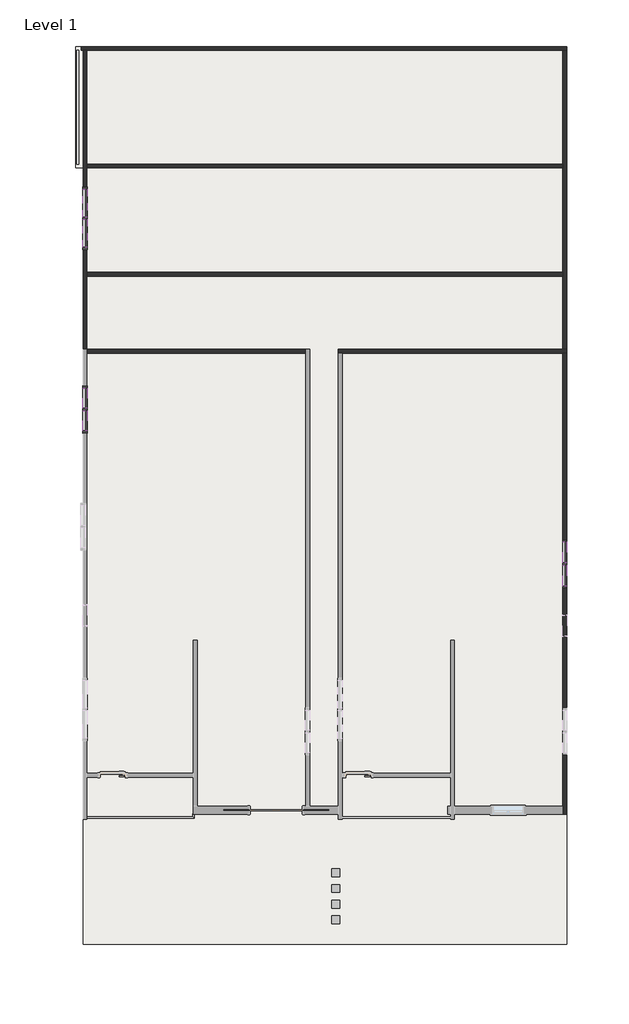
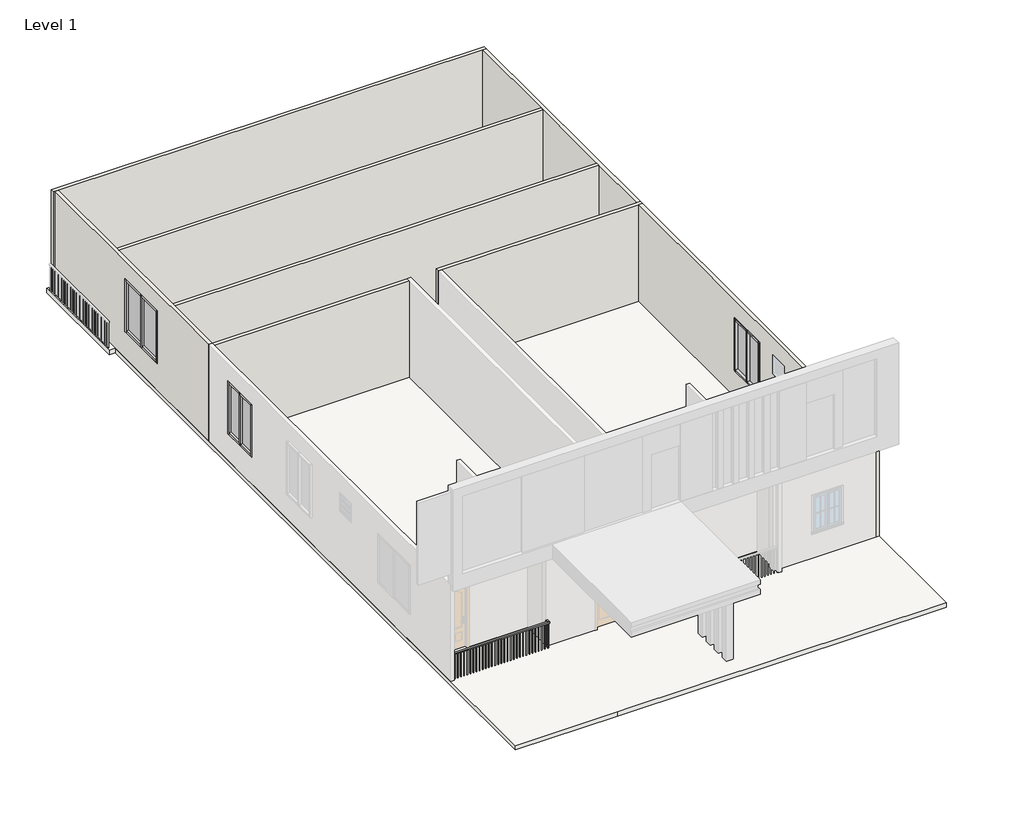
# One storey, part 2 of 3: 21 members, 8 walls, 6 plates, 1 railing, 1 slab.
"""IFC4 building model written with IfcOpenShell, lengths in millimetres."""

from ifc_helpers import new_model, si_unit, frame, origin, origin_with_axes, place, context, project, spatial, polyline, outline, extrude, faceted_brep, transform, mapped, element, save
from components import member_3f0e0172, member_96ae0c19, member_d60e8053, member_2fae0574, member_3e1d4a65, system_panel_glazed_c4393626, system_panel_glazed_d2c73f4b, system_panel_glazed_30879ba3

model = new_model("IFC4")

# Units and contexts
model_context = context("Model", 3, world=origin())
ifc_project = project(units=[si_unit("LENGTHUNIT", "METRE", prefix="MILLI")], contexts=[model_context])

# Site, building, storey
site = spatial("IfcSite", under=ifc_project)
building = spatial("IfcBuilding", under=site)
storey = spatial("IfcBuildingStorey", under=building, Name="Level 1", Elevation=0.0)

# Members
placement = place(None, origin())
member_shape = member_3f0e0172(model_context)
element("IfcMember", 1, ObjectType="Rectangular Mullion : 2.5\" x 5\" rectangular", at=placement, inside=storey, context=model_context, shape_type="MappedRepresentation", body=[
    mapped(member_shape, transform((5848.1708786, -3933.7021821, 2743.2), x_axis=(0.0, 0.0, 1.0), y_axis=(-1.0, 0.0, 0.0), z_axis=(0.0, -1.0, 0.0))),
])
element("IfcMember", 2, ObjectType="Rectangular Mullion : 2.5\" x 5\" rectangular", at=placement, inside=storey, context=model_context, shape_type="MappedRepresentation", body=[
    mapped(member_shape, transform((5848.1708786, -3254.2521821, 2743.2), x_axis=(0.0, 0.0, 1.0), y_axis=(-1.0, 0.0, 0.0), z_axis=(0.0, -1.0, 0.0))),
])
element("IfcMember", 3, ObjectType="Rectangular Mullion : 2.5\" x 5\" rectangular", at=placement, inside=storey, context=model_context, shape_type="MappedRepresentation", body=[
    mapped(member_shape, transform((5848.1708786, -2638.3021821, 914.4), x_axis=(0.0, 0.0, -1.0), y_axis=(-1.0, 0.0, 0.0), z_axis=(0.0, 1.0, 0.0))),
])
element("IfcMember", 4, ObjectType="Rectangular Mullion : 2.5\" x 5\" rectangular", at=placement, inside=storey, context=model_context, shape_type="MappedRepresentation", body=[
    mapped(member_shape, transform((5848.1708786, -3317.7521821, 914.4), x_axis=(0.0, 0.0, -1.0), y_axis=(-1.0, 0.0, 0.0), z_axis=(0.0, 1.0, 0.0))),
])
member_2_shape = member_96ae0c19(model_context)
element("IfcMember", 5, ObjectType="Rectangular Mullion : 2.5\" x 5\" rectangular", at=placement, inside=storey, context=model_context, shape_type="MappedRepresentation", body=[
    mapped(member_2_shape, transform((-8153.157583, 600.1666267, 2743.2), x_axis=(0.0, 0.0, 1.0), y_axis=(-1.0, 0.0, 0.0), z_axis=(0.0, -1.0, 0.0))),
])
element("IfcMember", 6, ObjectType="Rectangular Mullion : 2.5\" x 5\" rectangular", at=placement, inside=storey, context=model_context, shape_type="MappedRepresentation", body=[
    mapped(member_2_shape, transform((-8153.157583, 1254.9937905, 2743.2), x_axis=(0.0, 0.0, 1.0), y_axis=(-1.0, 0.0, 0.0), z_axis=(0.0, -1.0, 0.0))),
])
element("IfcMember", 7, ObjectType="Rectangular Mullion : 2.5\" x 5\" rectangular", at=placement, inside=storey, context=model_context, shape_type="MappedRepresentation", body=[
    mapped(member_2_shape, transform((-8153.157583, 1846.3209543, 914.4), x_axis=(0.0, 0.0, -1.0), y_axis=(-1.0, 0.0, 0.0), z_axis=(0.0, 1.0, 0.0))),
])
element("IfcMember", 8, ObjectType="Rectangular Mullion : 2.5\" x 5\" rectangular", at=placement, inside=storey, context=model_context, shape_type="MappedRepresentation", body=[
    mapped(member_2_shape, transform((-8153.157583, 1191.4937905, 914.4), x_axis=(0.0, 0.0, -1.0), y_axis=(-1.0, 0.0, 0.0), z_axis=(0.0, 1.0, 0.0))),
])
member_3_shape = member_d60e8053(model_context)
element("IfcMember", 9, ObjectType="Rectangular Mullion : 2.5\" x 5\" rectangular", at=placement, inside=storey, context=model_context, shape_type="MappedRepresentation", body=[
    mapped(member_3_shape, transform((5848.1708786, -3286.0021821, 914.4), x_axis=(0.0, -1.0, 0.0), y_axis=(-1.0, 0.0, 0.0), z_axis=(0.0, 0.0, -1.0))),
])
element("IfcMember", 10, ObjectType="Rectangular Mullion : 2.5\" x 5\" rectangular", at=placement, inside=storey, context=model_context, shape_type="MappedRepresentation", body=[
    mapped(member_3_shape, transform((-8153.157583, 1223.2437905, 914.4), x_axis=(0.0, -1.0, 0.0), y_axis=(-1.0, 0.0, 0.0), z_axis=(0.0, 0.0, -1.0))),
])
element("IfcMember", 11, ObjectType="Rectangular Mullion : 2.5\" x 5\" rectangular", at=placement, inside=storey, context=model_context, shape_type="MappedRepresentation", body=[
    mapped(member_3_shape, transform((-8153.157583, 6807.1511393, 914.4), x_axis=(0.0, -1.0, 0.0), y_axis=(-1.0, 0.0, 0.0), z_axis=(0.0, 0.0, -1.0))),
])
member_4_shape = member_2fae0574(model_context)
element("IfcMember", 12, ObjectType="Rectangular Mullion : 2.5\" x 5\" rectangular", at=placement, inside=storey, context=model_context, shape_type="MappedRepresentation", body=[
    mapped(member_4_shape, transform((5848.1708786, -2574.8021821, 2743.2), x_axis=(0.0, 1.0, 0.0), y_axis=(-1.0, 0.0, 0.0), z_axis=(0.0, 0.0, 1.0))),
])
element("IfcMember", 13, ObjectType="Rectangular Mullion : 2.5\" x 5\" rectangular", at=placement, inside=storey, context=model_context, shape_type="MappedRepresentation", body=[
    mapped(member_4_shape, transform((-8153.157583, 1909.8209543, 2743.2), x_axis=(0.0, 1.0, 0.0), y_axis=(-1.0, 0.0, 0.0), z_axis=(0.0, 0.0, 1.0))),
])
element("IfcMember", 14, ObjectType="Rectangular Mullion : 2.5\" x 5\" rectangular", at=placement, inside=storey, context=model_context, shape_type="MappedRepresentation", body=[
    mapped(member_4_shape, transform((-8153.157583, 7721.9533991, 2743.2), x_axis=(0.0, 1.0, 0.0), y_axis=(-1.0, 0.0, 0.0), z_axis=(0.0, 0.0, 1.0))),
])
element("IfcMember", 15, ObjectType="Rectangular Mullion : 2.5\" x 5\" rectangular", at=placement, inside=storey, context=model_context, shape_type="MappedRepresentation", body=[
    mapped(member_4_shape, transform((5848.1708786, -3997.2021821, 914.4), x_axis=(0.0, -1.0, 0.0), y_axis=(-1.0, 0.0, 0.0), z_axis=(0.0, 0.0, -1.0))),
])
element("IfcMember", 16, ObjectType="Rectangular Mullion : 2.5\" x 5\" rectangular", at=placement, inside=storey, context=model_context, shape_type="MappedRepresentation", body=[
    mapped(member_4_shape, transform((-8153.157583, 536.6666267, 914.4), x_axis=(0.0, -1.0, 0.0), y_axis=(-1.0, 0.0, 0.0), z_axis=(0.0, 0.0, -1.0))),
])
element("IfcMember", 17, ObjectType="Rectangular Mullion : 2.5\" x 5\" rectangular", at=placement, inside=storey, context=model_context, shape_type="MappedRepresentation", body=[
    mapped(member_4_shape, transform((-8153.157583, 5892.3488795, 914.4), x_axis=(0.0, -1.0, 0.0), y_axis=(-1.0, 0.0, 0.0), z_axis=(0.0, 0.0, -1.0))),
])
member_5_shape = member_3e1d4a65(model_context)
element("IfcMember", 18, ObjectType="Rectangular Mullion : 2.5\" x 5\" rectangular", at=placement, inside=storey, context=model_context, shape_type="MappedRepresentation", body=[
    mapped(member_5_shape, transform((-8153.157583, 5955.8488795, 2743.2), x_axis=(0.0, 0.0, 1.0), y_axis=(-1.0, 0.0, 0.0), z_axis=(0.0, -1.0, 0.0))),
])
element("IfcMember", 19, ObjectType="Rectangular Mullion : 2.5\" x 5\" rectangular", at=placement, inside=storey, context=model_context, shape_type="MappedRepresentation", body=[
    mapped(member_5_shape, transform((-8153.157583, 6838.9011393, 2743.2), x_axis=(0.0, 0.0, 1.0), y_axis=(-1.0, 0.0, 0.0), z_axis=(0.0, -1.0, 0.0))),
])
element("IfcMember", 20, ObjectType="Rectangular Mullion : 2.5\" x 5\" rectangular", at=placement, inside=storey, context=model_context, shape_type="MappedRepresentation", body=[
    mapped(member_5_shape, transform((-8153.157583, 7658.4533991, 914.4), x_axis=(0.0, 0.0, -1.0), y_axis=(-1.0, 0.0, 0.0), z_axis=(0.0, 1.0, 0.0))),
])
element("IfcMember", 21, ObjectType="Rectangular Mullion : 2.5\" x 5\" rectangular", at=placement, inside=storey, context=model_context, shape_type="MappedRepresentation", body=[
    mapped(member_5_shape, transform((-8153.157583, 6775.4011393, 914.4), x_axis=(0.0, 0.0, -1.0), y_axis=(-1.0, 0.0, 0.0), z_axis=(0.0, 1.0, 0.0))),
])

# Plates
system_panel_glazed_shape = system_panel_glazed_c4393626(model_context)
element("IfcPlate", 22, ObjectType="System Panel : Glazed", at=placement, inside=storey, context=model_context, shape_type="MappedRepresentation", body=[
    mapped(system_panel_glazed_shape, transform((-8153.157583, 1550.6573724, 977.9), x_axis=(0.0, -1.0, 0.0), y_axis=(1.0, 0.0, 0.0), z_axis=(0.0, 0.0, 1.0))),
])
element("IfcPlate", 23, ObjectType="System Panel : Glazed", at=placement, inside=storey, context=model_context, shape_type="MappedRepresentation", body=[
    mapped(system_panel_glazed_shape, transform((-8153.157583, 895.8302086, 977.9), x_axis=(0.0, -1.0, 0.0), y_axis=(1.0, 0.0, 0.0), z_axis=(0.0, 0.0, 1.0))),
])
system_panel_glazed_2_shape = system_panel_glazed_d2c73f4b(model_context)
element("IfcPlate", 24, ObjectType="System Panel : Glazed", at=placement, inside=storey, context=model_context, shape_type="MappedRepresentation", body=[
    mapped(system_panel_glazed_2_shape, transform((5848.1708786, -2946.2771821, 977.9), x_axis=(0.0, -1.0, 0.0), y_axis=(1.0, 0.0, 0.0), z_axis=(0.0, 0.0, 1.0))),
])
element("IfcPlate", 25, ObjectType="System Panel : Glazed", at=placement, inside=storey, context=model_context, shape_type="MappedRepresentation", body=[
    mapped(system_panel_glazed_2_shape, transform((5848.1708786, -3625.7271821, 977.9), x_axis=(0.0, -1.0, 0.0), y_axis=(1.0, 0.0, 0.0), z_axis=(0.0, 0.0, 1.0))),
])
system_panel_glazed_3_shape = system_panel_glazed_30879ba3(model_context)
element("IfcPlate", 26, ObjectType="System Panel : Glazed", at=placement, inside=storey, context=model_context, shape_type="MappedRepresentation", body=[
    mapped(system_panel_glazed_3_shape, transform((-8153.157583, 7248.6772692, 977.9), x_axis=(0.0, -1.0, 0.0), y_axis=(1.0, 0.0, 0.0), z_axis=(0.0, 0.0, 1.0))),
])
element("IfcPlate", 27, ObjectType="System Panel : Glazed", at=placement, inside=storey, context=model_context, shape_type="MappedRepresentation", body=[
    mapped(system_panel_glazed_3_shape, transform((-8153.157583, 6365.6250094, 977.9), x_axis=(0.0, -1.0, 0.0), y_axis=(1.0, 0.0, 0.0), z_axis=(0.0, 0.0, 1.0))),
])

# Railing
element("IfcRailing", 28, ObjectType="Handrail - Rectangular", at=placement, inside=storey, context=model_context, shape_type="SolidModel", body=[
    faceted_brep([(-8153.157583, -10659.0005933, 914.4), (-8153.157583, -10659.0005933, 863.6), (-8153.157583, -10709.8005933, 863.6), (-8153.157583, -10709.8005933, 914.4), (-5014.0237038, -10659.0005933, 914.4), (-5014.0237038, -10659.0005933, 863.6), (-4963.2237038, -10709.8005933, 863.6), (-4963.2237038, -10709.8005933, 914.4), (-5014.0237038, -10582.0742041, 914.4), (-4963.2237038, -10582.0742041, 914.4), (-4963.2237038, -10582.0742041, 863.6), (-5014.0237038, -10582.0742041, 863.6)], [[[0, 1, 2, 3]], [[1, 0, 4, 5]], [[2, 1, 5, 6]], [[3, 2, 6, 7]], [[0, 3, 7, 4]], [[8, 9, 10, 11]], [[5, 4, 8, 11]], [[6, 5, 11, 10]], [[7, 6, 10, 9]], [[4, 7, 9, 8]]]),
    extrude(outline(polyline([(-4979.0987038, -10592.3255933), (-4998.1487038, -10592.3255933), (-4998.1487038, -10573.2755933), (-4979.0987038, -10573.2755933), (-4979.0987038, -10592.3255933)])), origin_with_axes(), (0.0, 0.0, 1.0), 863.6),
    extrude(outline(polyline([(-5013.082583, -10693.9255933), (-5013.082583, -10674.8755933), (-4994.032583, -10674.8755933), (-4994.032583, -10693.9255933), (-5013.082583, -10693.9255933)])), origin_with_axes(), (0.0, 0.0, 1.0), 863.6),
    extrude(outline(polyline([(-5114.682583, -10693.9255933), (-5114.682583, -10674.8755933), (-5095.632583, -10674.8755933), (-5095.632583, -10693.9255933), (-5114.682583, -10693.9255933)])), origin_with_axes(), (0.0, 0.0, 1.0), 863.6),
    extrude(outline(polyline([(-5216.282583, -10693.9255933), (-5216.282583, -10674.8755933), (-5197.232583, -10674.8755933), (-5197.232583, -10693.9255933), (-5216.282583, -10693.9255933)])), origin_with_axes(), (0.0, 0.0, 1.0), 863.6),
    extrude(outline(polyline([(-5317.882583, -10693.9255933), (-5317.882583, -10674.8755933), (-5298.832583, -10674.8755933), (-5298.832583, -10693.9255933), (-5317.882583, -10693.9255933)])), origin_with_axes(), (0.0, 0.0, 1.0), 863.6),
    extrude(outline(polyline([(-5419.482583, -10693.9255933), (-5419.482583, -10674.8755933), (-5400.432583, -10674.8755933), (-5400.432583, -10693.9255933), (-5419.482583, -10693.9255933)])), origin_with_axes(), (0.0, 0.0, 1.0), 863.6),
    extrude(outline(polyline([(-5521.082583, -10693.9255933), (-5521.082583, -10674.8755933), (-5502.032583, -10674.8755933), (-5502.032583, -10693.9255933), (-5521.082583, -10693.9255933)])), origin_with_axes(), (0.0, 0.0, 1.0), 863.6),
    extrude(outline(polyline([(-5622.682583, -10693.9255933), (-5622.682583, -10674.8755933), (-5603.632583, -10674.8755933), (-5603.632583, -10693.9255933), (-5622.682583, -10693.9255933)])), origin_with_axes(), (0.0, 0.0, 1.0), 863.6),
    extrude(outline(polyline([(-5724.282583, -10693.9255933), (-5724.282583, -10674.8755933), (-5705.232583, -10674.8755933), (-5705.232583, -10693.9255933), (-5724.282583, -10693.9255933)])), origin_with_axes(), (0.0, 0.0, 1.0), 863.6),
    extrude(outline(polyline([(-5825.882583, -10693.9255933), (-5825.882583, -10674.8755933), (-5806.832583, -10674.8755933), (-5806.832583, -10693.9255933), (-5825.882583, -10693.9255933)])), origin_with_axes(), (0.0, 0.0, 1.0), 863.6),
    extrude(outline(polyline([(-5927.482583, -10693.9255933), (-5927.482583, -10674.8755933), (-5908.432583, -10674.8755933), (-5908.432583, -10693.9255933), (-5927.482583, -10693.9255933)])), origin_with_axes(), (0.0, 0.0, 1.0), 863.6),
    extrude(outline(polyline([(-6029.082583, -10693.9255933), (-6029.082583, -10674.8755933), (-6010.032583, -10674.8755933), (-6010.032583, -10693.9255933), (-6029.082583, -10693.9255933)])), origin_with_axes(), (0.0, 0.0, 1.0), 863.6),
    extrude(outline(polyline([(-6130.682583, -10693.9255933), (-6130.682583, -10674.8755933), (-6111.632583, -10674.8755933), (-6111.632583, -10693.9255933), (-6130.682583, -10693.9255933)])), origin_with_axes(), (0.0, 0.0, 1.0), 863.6),
    extrude(outline(polyline([(-6232.282583, -10693.9255933), (-6232.282583, -10674.8755933), (-6213.232583, -10674.8755933), (-6213.232583, -10693.9255933), (-6232.282583, -10693.9255933)])), origin_with_axes(), (0.0, 0.0, 1.0), 863.6),
    extrude(outline(polyline([(-6333.882583, -10693.9255933), (-6333.882583, -10674.8755933), (-6314.832583, -10674.8755933), (-6314.832583, -10693.9255933), (-6333.882583, -10693.9255933)])), origin_with_axes(), (0.0, 0.0, 1.0), 863.6),
    extrude(outline(polyline([(-6435.482583, -10693.9255933), (-6435.482583, -10674.8755933), (-6416.432583, -10674.8755933), (-6416.432583, -10693.9255933), (-6435.482583, -10693.9255933)])), origin_with_axes(), (0.0, 0.0, 1.0), 863.6),
    extrude(outline(polyline([(-6537.082583, -10693.9255933), (-6537.082583, -10674.8755933), (-6518.032583, -10674.8755933), (-6518.032583, -10693.9255933), (-6537.082583, -10693.9255933)])), origin_with_axes(), (0.0, 0.0, 1.0), 863.6),
    extrude(outline(polyline([(-6638.682583, -10693.9255933), (-6638.682583, -10674.8755933), (-6619.632583, -10674.8755933), (-6619.632583, -10693.9255933), (-6638.682583, -10693.9255933)])), origin_with_axes(), (0.0, 0.0, 1.0), 863.6),
    extrude(outline(polyline([(-6740.282583, -10693.9255933), (-6740.282583, -10674.8755933), (-6721.232583, -10674.8755933), (-6721.232583, -10693.9255933), (-6740.282583, -10693.9255933)])), origin_with_axes(), (0.0, 0.0, 1.0), 863.6),
    extrude(outline(polyline([(-6841.882583, -10693.9255933), (-6841.882583, -10674.8755933), (-6822.832583, -10674.8755933), (-6822.832583, -10693.9255933), (-6841.882583, -10693.9255933)])), origin_with_axes(), (0.0, 0.0, 1.0), 863.6),
    extrude(outline(polyline([(-6943.482583, -10693.9255933), (-6943.482583, -10674.8755933), (-6924.432583, -10674.8755933), (-6924.432583, -10693.9255933), (-6943.482583, -10693.9255933)])), origin_with_axes(), (0.0, 0.0, 1.0), 863.6),
    extrude(outline(polyline([(-7045.082583, -10693.9255933), (-7045.082583, -10674.8755933), (-7026.032583, -10674.8755933), (-7026.032583, -10693.9255933), (-7045.082583, -10693.9255933)])), origin_with_axes(), (0.0, 0.0, 1.0), 863.6),
    extrude(outline(polyline([(-7146.682583, -10693.9255933), (-7146.682583, -10674.8755933), (-7127.632583, -10674.8755933), (-7127.632583, -10693.9255933), (-7146.682583, -10693.9255933)])), origin_with_axes(), (0.0, 0.0, 1.0), 863.6),
    extrude(outline(polyline([(-7248.282583, -10693.9255933), (-7248.282583, -10674.8755933), (-7229.232583, -10674.8755933), (-7229.232583, -10693.9255933), (-7248.282583, -10693.9255933)])), origin_with_axes(), (0.0, 0.0, 1.0), 863.6),
    extrude(outline(polyline([(-7349.882583, -10693.9255933), (-7349.882583, -10674.8755933), (-7330.832583, -10674.8755933), (-7330.832583, -10693.9255933), (-7349.882583, -10693.9255933)])), origin_with_axes(), (0.0, 0.0, 1.0), 863.6),
    extrude(outline(polyline([(-7451.482583, -10693.9255933), (-7451.482583, -10674.8755933), (-7432.432583, -10674.8755933), (-7432.432583, -10693.9255933), (-7451.482583, -10693.9255933)])), origin_with_axes(), (0.0, 0.0, 1.0), 863.6),
    extrude(outline(polyline([(-7553.082583, -10693.9255933), (-7553.082583, -10674.8755933), (-7534.032583, -10674.8755933), (-7534.032583, -10693.9255933), (-7553.082583, -10693.9255933)])), origin_with_axes(), (0.0, 0.0, 1.0), 863.6),
    extrude(outline(polyline([(-7654.682583, -10693.9255933), (-7654.682583, -10674.8755933), (-7635.632583, -10674.8755933), (-7635.632583, -10693.9255933), (-7654.682583, -10693.9255933)])), origin_with_axes(), (0.0, 0.0, 1.0), 863.6),
    extrude(outline(polyline([(-7756.282583, -10693.9255933), (-7756.282583, -10674.8755933), (-7737.232583, -10674.8755933), (-7737.232583, -10693.9255933), (-7756.282583, -10693.9255933)])), origin_with_axes(), (0.0, 0.0, 1.0), 863.6),
    extrude(outline(polyline([(-7857.882583, -10693.9255933), (-7857.882583, -10674.8755933), (-7838.832583, -10674.8755933), (-7838.832583, -10693.9255933), (-7857.882583, -10693.9255933)])), origin_with_axes(), (0.0, 0.0, 1.0), 863.6),
    extrude(outline(polyline([(-7959.482583, -10693.9255933), (-7959.482583, -10674.8755933), (-7940.432583, -10674.8755933), (-7940.432583, -10693.9255933), (-7959.482583, -10693.9255933)])), origin_with_axes(), (0.0, 0.0, 1.0), 863.6),
    extrude(outline(polyline([(-8061.082583, -10693.9255933), (-8061.082583, -10674.8755933), (-8042.032583, -10674.8755933), (-8042.032583, -10693.9255933), (-8061.082583, -10693.9255933)])), origin_with_axes(), (0.0, 0.0, 1.0), 863.6),
    extrude(outline(polyline([(-4998.1487038, -10693.9255933), (-4998.1487038, -10674.8755933), (-4979.0987038, -10674.8755933), (-4979.0987038, -10693.9255933), (-4998.1487038, -10693.9255933)])), origin_with_axes(), (0.0, 0.0, 1.0), 863.6),
    extrude(outline(polyline([(-4979.0987038, -10601.1242041), (-4998.1487038, -10601.1242041), (-4998.1487038, -10582.0742041), (-4979.0987038, -10582.0742041), (-4979.0987038, -10601.1242041)])), origin_with_axes(), (0.0, 0.0, 1.0), 863.6),
    extrude(outline(polyline([(-8153.157583, -10693.9255933), (-8153.157583, -10674.8755933), (-8134.107583, -10674.8755933), (-8134.107583, -10693.9255933), (-8153.157583, -10693.9255933)])), origin_with_axes(), (0.0, 0.0, 1.0), 863.6),
])

# Slab
element("IfcSlab", 29, ObjectType="6\" floor", at=placement, inside=storey, context=model_context, shape_type="SweptSolid", body=[
    extrude(outline(polyline([(5905.3208786, 11818.2189683), (5905.3208786, -14391.4493641), (-4874.3237038, -14391.4493641), (-8210.307583, -14391.4493641), (-8210.307583, 8277.3011327), (-8419.607647, 8277.3011327), (-8419.607647, 11818.2189683), (5905.3208786, 11818.2189683)])), frame((0.0, 0.0, -152.4), z_axis=(0.0, 0.0, 1.0), x_axis=(1.0, 0.0, 0.0)), (0.0, 0.0, 1.0), 152.4),
])

# Walls
element("IfcWall", 30, ObjectType="4.5\" wall", at=placement, inside=storey, context=model_context, shape_type="Brep", body=[
    faceted_brep([(-8267.457583, 11703.9189683, 0.0), (-8210.307583, 11703.9189683, 0.0), (-8096.007583, 11703.9189683, 0.0), (5791.0208786, 11703.9189683, 0.0), (5905.3208786, 11703.9189683, 0.0), (5905.3208786, 11703.9189683, 3352.8), (5791.0208786, 11703.9189683, 3352.8), (-8096.007583, 11703.9189683, 3352.8), (-8210.307583, 11703.9189683, 3352.8), (-8267.457583, 11703.9189683, 3352.8), (-8267.457583, 11818.2189683, 0.0), (-8267.457583, 11818.2189683, 3352.8), (5905.3208786, 11818.2189683, 3352.8), (5905.3208786, 11818.2189683, 0.0)], [[[0, 1, 2, 3, 4, 5, 6, 7, 8, 9]], [[10, 11, 12, 13]], [[4, 3, 2, 1, 0, 10, 13]], [[9, 8, 7, 6, 5, 12, 11]], [[0, 9, 11, 10]], [[5, 4, 13, 12]]]),
])
element("IfcWall", 31, ObjectType="4.5\" wall", at=placement, inside=storey, context=model_context, shape_type="Brep", body=[
    faceted_brep([(5791.0208786, 11703.9189683, 0.0), (5791.0208786, 8387.4224771, 0.0), (5791.0208786, 8273.1224771, 0.0), (5791.0208786, 5226.5048975, 0.0), (5791.0208786, 5112.2048975, 0.0), (5791.0208786, 2978.3002499, 0.0), (5791.0208786, 2978.3002499, 3352.8), (5791.0208786, 5112.2048975, 3352.8), (5791.0208786, 5226.5048975, 3352.8), (5791.0208786, 8273.1224771, 3352.8), (5791.0208786, 8387.4224771, 3352.8), (5791.0208786, 11703.9189683, 3352.8), (5905.3208786, 11703.9189683, 0.0), (5905.3208786, 11703.9189683, 3352.8), (5905.3208786, 2978.3002499, 3352.8), (5905.3208786, 2978.3002499, 0.0)], [[[0, 1, 2, 3, 4, 5, 6, 7, 8, 9, 10, 11]], [[12, 13, 14, 15]], [[5, 4, 3, 2, 1, 0, 12, 15]], [[11, 10, 9, 8, 7, 6, 14, 13]], [[0, 11, 13, 12]], [[6, 5, 15, 14]]]),
])
element("IfcWall", 32, ObjectType="4.5\" wall", at=placement, inside=storey, context=model_context, shape_type="SweptSolid", body=[
    extrude(outline(polyline([(-1713.5935762, 2864.0002499), (-8096.007583, 2864.0002499), (-8096.007583, 2978.3002499), (-1713.5935762, 2978.3002499), (-1713.5935762, 2864.0002499)])), origin_with_axes(), (0.0, 0.0, 1.0), 3352.8),
])
element("IfcWall", 33, ObjectType="4.5\" wall", at=placement, inside=storey, context=model_context, shape_type="SweptSolid", body=[
    extrude(outline(polyline([(-8096.007583, 5226.5048975), (5791.0208786, 5226.5048975), (5791.0208786, 5112.2048975), (-8096.007583, 5112.2048975), (-8096.007583, 5226.5048975)])), origin_with_axes(), (0.0, 0.0, 1.0), 3352.8),
])
element("IfcWall", 34, ObjectType="4.5\" wall", at=placement, inside=storey, context=model_context, shape_type="SweptSolid", body=[
    extrude(outline(polyline([(-8096.007583, 8387.4224771), (5791.0208786, 8387.4224771), (5791.0208786, 8273.1224771), (-8096.007583, 8273.1224771), (-8096.007583, 8387.4224771)])), origin_with_axes(), (0.0, 0.0, 1.0), 3352.8),
])
element("IfcWall", 35, ObjectType="4.5\" wall", at=placement, inside=storey, context=model_context, shape_type="Brep", body=[
    faceted_brep([(-8096.007583, 2978.3002499, 0.0), (-8096.007583, 5112.2048975, 0.0), (-8096.007583, 5226.5048975, 0.0), (-8096.007583, 8273.1224771, 0.0), (-8096.007583, 8387.4224771, 0.0), (-8096.007583, 11703.9189683, 0.0), (-8096.007583, 11703.9189683, 3352.8), (-8096.007583, 8387.4224771, 3352.8), (-8096.007583, 8273.1224771, 3352.8), (-8096.007583, 5226.5048975, 3352.8), (-8096.007583, 5112.2048975, 3352.8), (-8096.007583, 2978.3002499, 3352.8), (-8096.007583, 7721.9533991, 2743.2), (-8096.007583, 7721.9533991, 914.4), (-8096.007583, 5892.3488795, 914.4), (-8096.007583, 5892.3488795, 2743.2), (-8210.307583, 11703.9189683, 0.0), (-8210.307583, 2978.3002499, 0.0), (-8210.307583, 2978.3002499, 3352.8), (-8210.307583, 11703.9189683, 3352.8), (-8210.307583, 7721.9533991, 914.4), (-8210.307583, 7721.9533991, 2743.2), (-8210.307583, 5892.3488795, 2743.2), (-8210.307583, 5892.3488795, 914.4)], [[[0, 1, 2, 3, 4, 5, 6, 7, 8, 9, 10, 11], [12, 13, 14, 15]], [[16, 17, 18, 19], [20, 21, 22, 23]], [[5, 4, 3, 2, 1, 0, 17, 16]], [[11, 10, 9, 8, 7, 6, 19, 18]], [[6, 5, 16, 19]], [[0, 11, 18, 17]], [[20, 13, 12, 21]], [[21, 12, 15, 22]], [[22, 15, 14, 23]], [[13, 20, 23, 14]]]),
])
element("IfcWall", 36, ObjectType="4.5\" wall", at=placement, inside=storey, context=model_context, shape_type="Brep", body=[
    faceted_brep([(5791.0208786, 2864.0002499, 0.0), (5791.0208786, -10357.2779557, 0.0), (5791.0208786, -10585.8779557, 0.0), (5791.0208786, -10585.8779557, 3352.8), (5791.0208786, -10357.2779557, 3352.8), (5791.0208786, 2864.0002499, 3352.8), (5791.0208786, -7489.2492493, 914.4), (5791.0208786, -7489.2492493, 2743.2), (5791.0208786, -8858.5998253, 2743.2), (5791.0208786, -8858.5998253, 914.4), (5791.0208786, -2574.8021821, 914.4), (5791.0208786, -2574.8021821, 2743.2), (5791.0208786, -3997.2021821, 2743.2), (5791.0208786, -3997.2021821, 914.4), (5791.0208786, -4784.6021821, 2762.25), (5791.0208786, -5394.2021821, 2762.25), (5791.0208786, -5394.2021821, 2152.65), (5791.0208786, -4784.6021821, 2152.65), (5905.3208786, -10585.8779557, 0.0), (5905.3208786, 2864.0002499, 0.0), (5905.3208786, 2864.0002499, 3352.8), (5905.3208786, -10585.8779557, 3352.8), (5905.3208786, -7489.2492493, 2743.2), (5905.3208786, -7489.2492493, 914.4), (5905.3208786, -8858.5998253, 914.4), (5905.3208786, -8858.5998253, 2743.2), (5905.3208786, -2574.8021821, 2743.2), (5905.3208786, -2574.8021821, 914.4), (5905.3208786, -3997.2021821, 914.4), (5905.3208786, -3997.2021821, 2743.2), (5905.3208786, -4784.6021821, 2762.25), (5905.3208786, -4784.6021821, 2152.65), (5905.3208786, -5394.2021821, 2152.65), (5905.3208786, -5394.2021821, 2762.25)], [[[0, 1, 2, 3, 4, 5], [6, 7, 8, 9], [10, 11, 12, 13], [14, 15, 16, 17]], [[18, 19, 20, 21], [22, 23, 24, 25], [26, 27, 28, 29], [30, 31, 32, 33]], [[2, 1, 0, 19, 18]], [[5, 4, 3, 21, 20]], [[0, 5, 20, 19]], [[3, 2, 18, 21]], [[6, 23, 22, 7]], [[7, 22, 25, 8]], [[8, 25, 24, 9]], [[23, 6, 9, 24]], [[26, 11, 10, 27]], [[11, 26, 29, 12]], [[12, 29, 28, 13]], [[27, 10, 13, 28]], [[31, 30, 14, 17]], [[32, 31, 17, 16]], [[33, 32, 16, 15]], [[30, 33, 15, 14]]]),
])
element("IfcWall", 37, ObjectType="4.5\" wall", at=placement, inside=storey, context=model_context, shape_type="Brep", body=[
    faceted_brep([(-762.8431282, 2864.0002499, 0.0), (-648.5431282, 2864.0002499, 0.0), (5791.0208786, 2864.0002499, 0.0), (5905.3208786, 2864.0002499, 0.0), (5905.3208786, 2864.0002499, 3352.8), (5791.0208786, 2864.0002499, 3352.8), (-648.5431282, 2864.0002499, 3352.8), (-762.8431282, 2864.0002499, 3352.8), (-762.8431282, 2978.3002499, 0.0), (-762.8431282, 2978.3002499, 3352.8), (5791.0208786, 2978.3002499, 3352.8), (5905.3208786, 2978.3002499, 3352.8), (5905.3208786, 2978.3002499, 0.0), (5791.0208786, 2978.3002499, 0.0)], [[[0, 1, 2, 3, 4, 5, 6, 7]], [[8, 9, 10, 11, 12, 13]], [[3, 2, 1, 0, 8, 13, 12]], [[7, 6, 5, 4, 11, 10, 9]], [[0, 7, 9, 8]], [[4, 3, 12, 11]]]),
])

save(model, "model.ifc")

# Revit data of these elements
# Type "Rectangular Mullion : 2.5\" x 5\" rectangular"
#   built-in parameter 1007304 = 0.416667 (stored number, unit not read)
#   built-in parameter 1007301 = 0.104167 (stored number, unit not read)
#   built-in parameter 1007300 = 0.104167 (stored number, unit not read)
# Type "System Panel : Glazed"
#   Construction Type Id = "GSP4R"
#   Analytic Construction = "1/8 in Pilkington single glazing"
#   Visual Light Transmittance = 0.9
#   Solar Heat Gain Coefficient = 0.86
#   Heat Transfer Coefficient (U) = 1.18115 BTU/(h·ft²·°F)
#   Define Thermal Properties by = 1
# Type "Handrail - Rectangular"
#   Assembly Code = "C2010400"
#   built-in parameter 1008612 = 0.0416667 (stored number, unit not read)
#   built-in parameter 1008611 = 0.0416667 (stored number, unit not read)
#   built-in parameter 1008609 = 0.333333 (stored number, unit not read)
#   built-in parameter 1008604 = 0.166667 (stored number, unit not read)
#   built-in parameter 1008603 = 0.166667 (stored number, unit not read)
#   Railing Height = 3' - 0"
#   built-in parameter 1008630 = 2
#   built-in parameter 1008610 = 2
#   built-in parameter 1008618 = Baluster - Square : 3/4"
# Type "6\" floor"
#   Assembly Code = "B1010"
#   Function = 0
#   Layers, outside or top first: 0' - 6" no material (function 1)
# Type "4.5\" wall"
#   Assembly Code = "B2010"
#   Layers, outside or top first: 0' - 4 1/2" no material (function 1)
# Elements 1, 2, 3, 4, 5, 6, 7, 8, 9, 10, 11, 12, 13, 14, 15, 16, 17, 18, 19, 20, 21 (IfcMember, "Rectangular Mullion : 2.5\" x 5\" rectangular")
#   Phase Created = New Construction
#   Materials on its faces: "Aluminum"
# Elements 22, 23, 24, 25, 26, 27 (IfcPlate, "System Panel : Glazed")
#   Phase Created = New Construction
#   Materials on its faces: "Glass"
# Element 28 (IfcRailing, "Handrail - Rectangular")
#   Phase Created = New Construction
# Element 29 (IfcSlab, "6\" floor")
#   Height Offset From Level = 0' - 0"
#   Phase Created = New Construction
#   Materials on its faces: "Default Floor"
# Elements 30, 31, 32, 33, 34, 35, 36, 37 (IfcWall, "4.5\" wall")
#   Top Offset = 0' - 0"
#   Base Offset = 0' - 0"
#   wall height = 11' - 0"
#   Phase Created = New Construction
#   Base Constraint = Level 1
#   Top Constraint = Level 2
#   Materials on its faces: "Default Wall"
# Materials
#   "Aluminum": class "Metal", colour RGB 247 247 247, transparency 0, Description = "Aluminum 6061", Cost = 0
#   "Glass": class "Glass", colour RGB 0 128 192, transparency 0.75, Description = "Soda Lime Glass", Cost = 0
#   "Default Floor": colour RGB 128 128 128, transparency 0, Cost = 0
#   "Default Wall": colour RGB 128 128 128, transparency 0, Cost = 0
